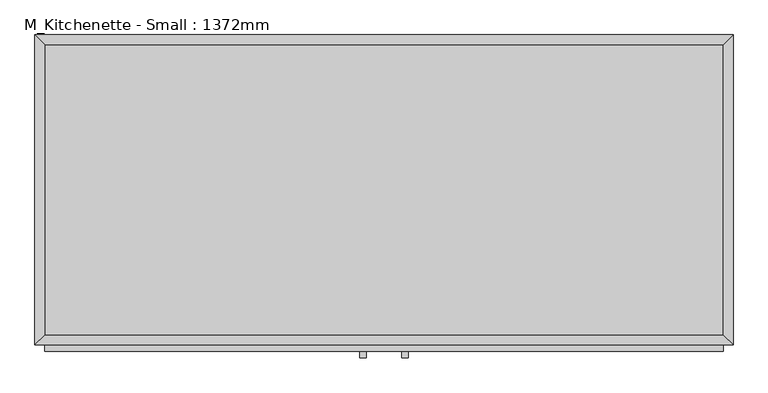
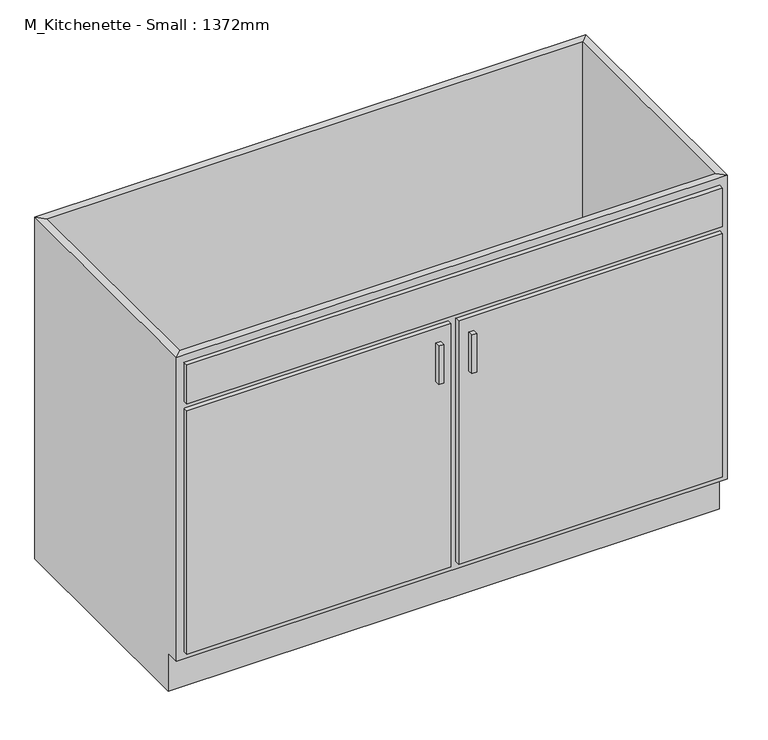
"""IFC4 building model written with IfcOpenShell, lengths in millimetres: proxy geometry, M_Kitchenette - Small : 1372mm."""

from ifc_helpers import new_model, si_unit, frame, origin, place, context, project, spatial, polyline, outline, extrude, faceted_brep, source, transform, mapped, element, save


def m_kitchenette_small_1372mm_f81b7602(model_context):
    return source(origin(), model_context, "Body", "SolidModel", [
        faceted_brep([(685.6877049, -590.95, 900.0), (685.6877049, -590.95, 100.0), (-648.2122951, -590.95, 100.0), (-648.2122951, -590.95, 900.0), (-667.2622951, -610.0, 900.0), (704.7377049, -610.0, 900.0), (-667.2622951, -610.0, 100.0), (704.7377049, -610.0, 100.0), (-648.2122951, -575.0, 100.0), (-648.2122951, -19.05, 100.0), (-648.2122951, -19.05, 900.0), (-667.2622951, 0.0, 900.0), (-667.2622951, 0.0, 0.0), (-667.2622951, -575.0, 0.0), (-667.2622951, -575.0, 100.0), (685.6877049, -19.05, 100.0), (685.6877049, -19.05, 900.0), (704.7377049, 0.0, 900.0), (704.7377049, 0.0, 0.0), (685.6877049, -575.0, 100.0), (704.7377049, -575.0, 100.0), (704.7377049, -575.0, 0.0)], [[[0, 1, 2, 3]], [[0, 3, 4, 5]], [[5, 4, 6, 7]], [[2, 1, 7, 6]], [[3, 2, 8, 9, 10]], [[4, 3, 10, 11]], [[6, 4, 11, 12, 13, 14]], [[2, 6, 14, 8]], [[10, 9, 15, 16]], [[11, 10, 16, 17]], [[12, 11, 17, 18]], [[1, 0, 16, 15, 19]], [[0, 5, 17, 16]], [[5, 7, 20, 21, 18, 17]], [[7, 1, 19, 20]], [[8, 19, 15, 9]], [[18, 21, 13, 12]], [[13, 21, 20, 19, 8, 14]]]),
        extrude(outline(polyline([(-16.1872951, -635.4), (-28.8872951, -635.4), (-28.8872951, -622.7), (-16.1872951, -622.7), (-16.1872951, -635.4)])), frame((0.0, 0.0, 620.6), z_axis=(0.0, 0.0, 1.0), x_axis=(1.0, 0.0, 0.0)), (0.0, 0.0, 1.0), 101.6),
        extrude(outline(polyline([(66.3627049, -635.4), (53.6627049, -635.4), (53.6627049, -622.7), (66.3627049, -622.7), (66.3627049, -635.4)])), frame((0.0, 0.0, 620.6), z_axis=(0.0, 0.0, 1.0), x_axis=(1.0, 0.0, 0.0)), (0.0, 0.0, 1.0), 101.6),
        extrude(outline(polyline([(9.2127049, -622.7), (-648.2122951, -622.7), (-648.2122951, -610.0), (9.2127049, -610.0), (9.2127049, -622.7)])), frame((0.0, 0.0, 119.05), z_axis=(0.0, 0.0, 1.0), x_axis=(1.0, 0.0, 0.0)), (0.0, 0.0, 1.0), 641.25),
        extrude(outline(polyline([(685.6877049, -622.7), (28.2627049, -622.7), (28.2627049, -610.0), (685.6877049, -610.0), (685.6877049, -622.7)])), frame((0.0, 0.0, 119.05), z_axis=(0.0, 0.0, 1.0), x_axis=(1.0, 0.0, 0.0)), (0.0, 0.0, 1.0), 641.25),
        extrude(outline(polyline([(685.6877049, -622.7), (-648.2122951, -622.7), (-648.2122951, -610.0), (685.6877049, -610.0), (685.6877049, -622.7)])), frame((0.0, 0.0, 779.35), z_axis=(0.0, 0.0, 1.0), x_axis=(1.0, 0.0, 0.0)), (0.0, 0.0, 1.0), 101.6),
        extrude(outline(polyline([(685.6877049, -19.05), (685.6877049, -590.95), (-648.2122951, -590.95), (-648.2122951, -19.05), (685.6877049, -19.05)])), frame((0.0, 0.0, 100.0), z_axis=(0.0, 0.0, 1.0), x_axis=(1.0, 0.0, 0.0)), (0.0, 0.0, 1.0), 19.05),
    ])


if __name__ == "__main__":
    model = new_model("IFC4")
    model_context = context("Model", 3, world=origin())
    ifc_project = project(units=[si_unit("LENGTHUNIT", "METRE", prefix="MILLI")], contexts=[model_context])
    site = spatial("IfcSite", under=ifc_project)
    building = spatial("IfcBuilding", under=site)
    placement = place(None, origin())
    m_kitchenette_small_1372mm_shape = m_kitchenette_small_1372mm_f81b7602(model_context)
    element("IfcBuildingElementProxy", 1, Name="M_Kitchenette - Small : 1372mm", ObjectType="M_Kitchenette - Small : 1372mm", at=placement, inside=building, context=model_context, shape_type="MappedRepresentation", body=[
        mapped(m_kitchenette_small_1372mm_shape, transform((0.0, 0.0, 0.0), x_axis=(1.0, 0.0, 0.0), y_axis=(0.0, 1.0, 0.0), z_axis=(0.0, 0.0, 1.0))),
    ])
    save(model, "model.ifc")

# Revit data of these elements
# Type "M_Kitchenette - Small : 1372mm"
#   Width = 1372 mm
#   Height = 900 mm
#   Depth = 610 mm
#   Toe Depth = 35 mm
#   Toe Height = 100 mm
#   Cabinet Material = Cabinets
#   Door/Drawer Material = Cabinets
#   Handle Material = Cabinets - Handles
#   Default Elevation = 0
# Element 1 (IfcBuildingElementProxy, "M_Kitchenette - Small : 1372mm")
#   Materials on its faces: "Cabinets", "Cabinets - Handles"
# Materials
#   "Cabinets": colour RGB 249 249 249, transparency 0
#   "Cabinets - Handles": class "Metal", colour RGB 57 57 57, transparency 0
